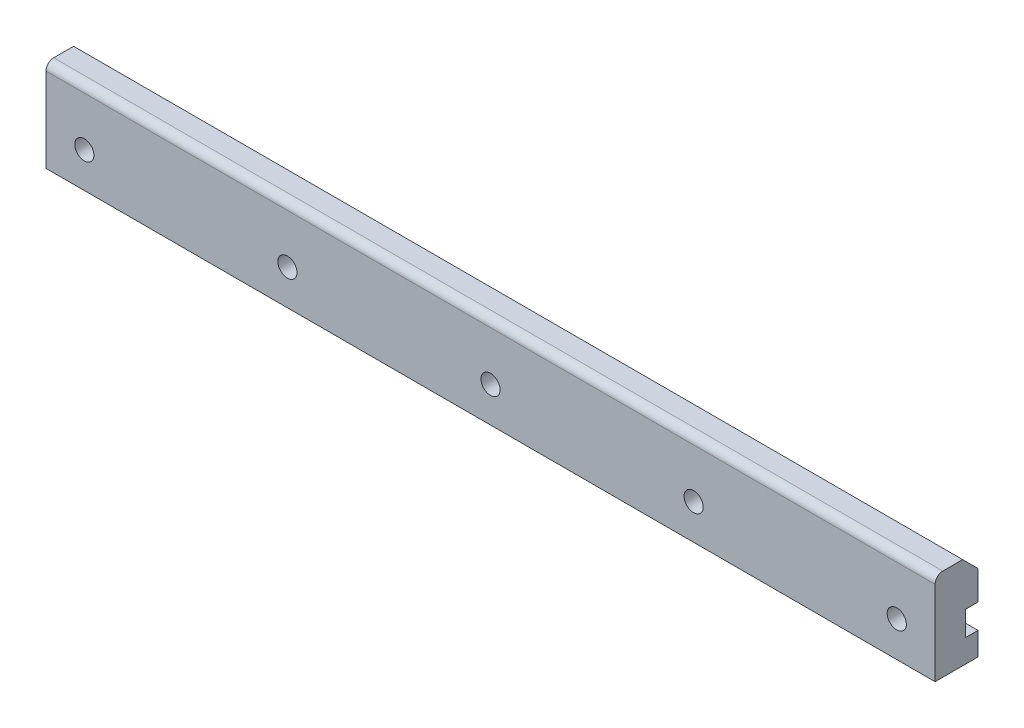
SolidWorks part; units mm, degrees
material "Plain Carbon Steel"
ref_plane "Front Plane" through (0, 0, 0) normal (0, 0, 1) x (1, 0, 0)
ref_plane "Top Plane" through (0, 0, 0) normal (0, 1, 0) x (1, 0, 0)
ref_plane "Right Plane" through (0, 0, 0) normal (1, 0, 0) x (0, 0, -1)
sketch "Rail Profile Sketch" plane through (0, 0, 0) normal (0, 0, 1) x (1, 0, 0)
  line L1 (-290, 30) -> (290, 30)
  line L2 (-290, 30) -> (-290, -30)
  line L3 (-290, -30) -> (290, -30)
  line L4 (290, 30) -> (290, -30)
  line L5 (-290, 30) -> (290, -30) construction
  line L6 (-290, -30) -> (290, 30) construction
  point P0 (0, 0)
  dimension "D1" = 60
  dimension "D2" = 580
extrude "Rail Bar 580x60x28" add sketch "Rail Profile Sketch" along normal blind 28
fillet "Edge Fillet R5" radius 5 1 edges at (0, 30, 28)
sketch "Groove Sketch" plane through (290, 0, 0) normal (1, 0, 0) x (0, 0, -1)
  line L0 (0, -30) -> (0, 30) construction
  line L1 (-8, 1) -> (8, 1)
  line L2 (-8, 1) -> (-8, -15)
  line L3 (-8, -15) -> (8, -15)
  line L4 (8, 1) -> (8, -15)
  line L5 (-8, 1) -> (8, -15) construction
  line L6 (-8, -15) -> (8, 1) construction
  line L8 (-28, -30) -> (0, -30) construction
  point P0 (0, -7)
  dimension "D1" = 16
  dimension "D2" = 16
  dimension "D3" = 15
extrude "Longitudinal Groove 16x16" cut sketch "Groove Sketch" against normal through all
chamfer "Edge Chamfer 10x45" distance 10 angle 45 1 edges at (0, 30, 0)
sketch "Mounting Holes Sketch" plane through (0, 0, 28) normal (0, 0, 1) x (1, 0, 0)
  line L0 (-290, 25) -> (-290, -30) construction
  line L1 (-290, -30) -> (290, -30) construction
  line L2 (-265, -7) -> (-132.5, -7) construction
  circle A0 centre (-265, -7) radius 6.25
  circle A1 centre (-132.5, -7) radius 6.25
  circle A2 centre (0, -7) radius 6.25
  circle A3 centre (132.5, -7) radius 6.25
  circle A4 centre (265, -7) radius 6.25
  dimension "D1" = 12.5
  dimension "D2" = 25
  dimension "D3" = 23
  dimension "D5" = 132.5
  dimension "D4" = 5
extrude "Mounting Holes 5x" cut sketch "Mounting Holes Sketch" against normal through all contours A1
